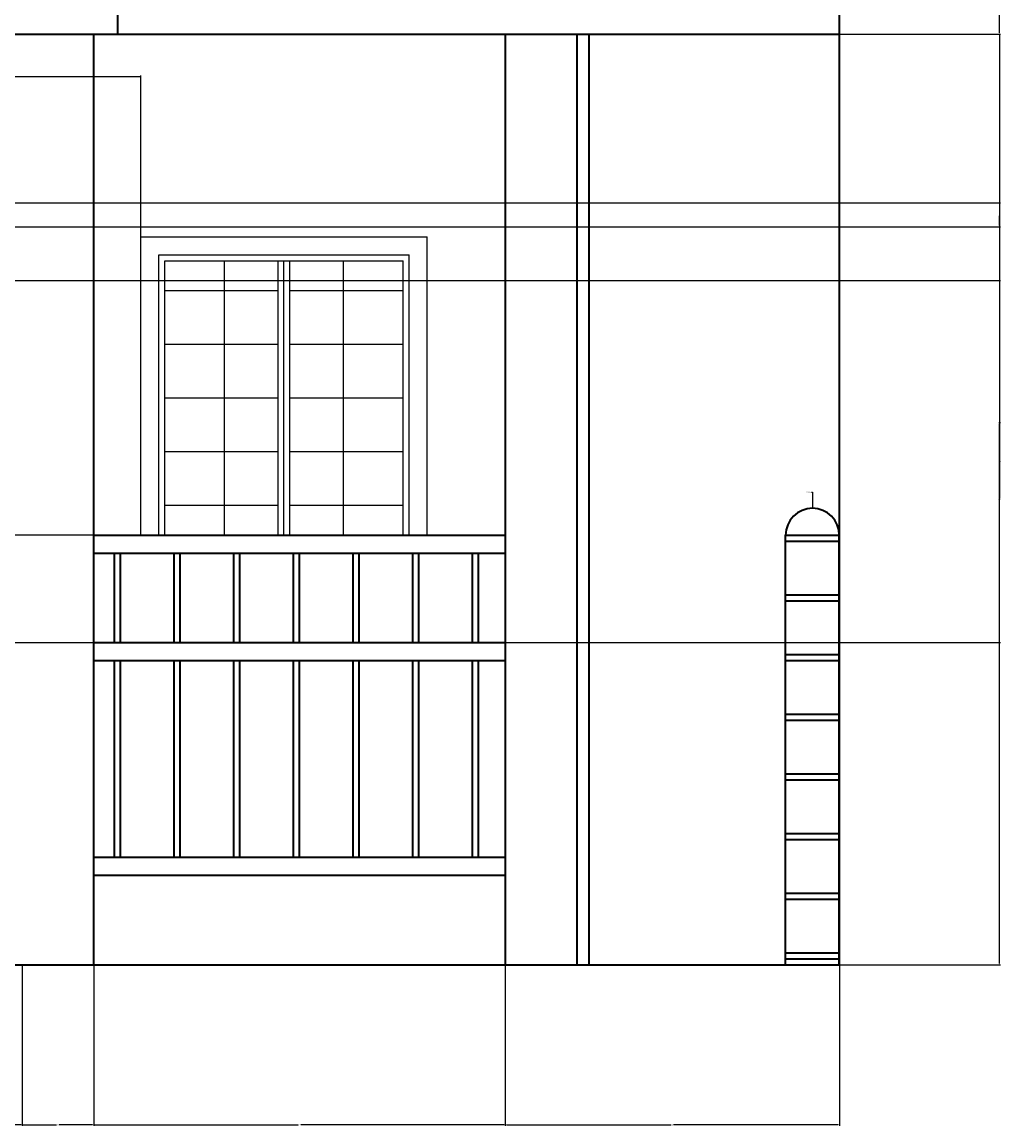
# Model space of a CAD drawing. Units: inches. Extents: x 2154 to 2740, y 571 to 1084.
# Tile 7 of 13: x 2576 to 2740, y 571 to 756. Entities that reach past the tile are written whole.
import ezdxf

# ---------------------------------------------------------------- set-up
doc = ezdxf.new("R2010")
doc.units = ezdxf.units.IN
for name, color, linetype, lineweight in [('A-ANNO-DIMS', 2, 'Continuous', 18), ('A-ELEV', 7, 'Continuous', 35), ('A-GLAZ', 4, 'Continuous', 25)]:
    doc.layers.add(name, color=color, linetype=linetype, lineweight=lineweight)
doc.styles.get("Standard").update_dxf_attribs({"font": 'arial.ttf'})
doc.dimstyles.get("Standard").update_dxf_attribs({"dimtxt": 0.18, "dimasz": 0.18, "dimexe": 0.18, "dimexo": 0.0625, "dimgap": 0.09, "dimtad": 0, "dimtih": 1, "dimtoh": 1, "dimdec": 4, "dimzin": 0, "dimdsep": 46, "dimtxsty": 'Standard', "dimcen": 0.09, "dimadec": 0, "dimazin": 0, "dimtfac": 1, "dimtdec": 4, "dimtofl": 0, "dimtmove": 0, "dimatfit": 3, "dimfxl": 1, "dimtolj": 1, "dimtzin": 0, "dimarcsym": 0})

# ---------------------------------------------------------------- blocks, each defined once
blk = doc.blocks.new('WIN-ELEV-1200')
for p, q in [((0, 50), (48, 50)), ((0, 0), (0, 50)), ((48, 0), (48, 50)), ((3, 0), (3, 47)), ((3, 47), (45, 47)), ((45, 0), (45, 47)), ((4, 46), (44, 46)), ((4, 0), (4, 46)), ((14, 0), (14, 46)), ((23, 0), (23, 46)), ((24, 0), (24, 46)), ((25, 0), (25, 46)), ((34, 0), (34, 46)), ((44, 0), (44, 46)), ((4, 41), (23, 41)), ((25, 41), (44, 41)), ((4, 32), (23, 32)), ((25, 32), (44, 32)), ((4, 23), (23, 23)), ((25, 23), (44, 23)), ((4, 14), (23, 14)), ((25, 14), (44, 14)), ((4, 5), (23, 5)), ((25, 5), (44, 5))]:
    blk.add_line(p, q)
blk = doc.blocks.new('*D11')
at = {"layer": 'A-ANNO-DIMS', "color": 0, "lineweight": -2, "transparency": 16777216}
for p, q in [((2713.27, 753.53), (2740.24, 753.53)), ((2740.06, 753.35), (2740.06, 675.71)), ((2740.06, 597.71), (2740.06, 675.35)), ((2713.27, 597.53), (2740.24, 597.53))]:
    blk.add_line(p, q, dxfattribs=at)
at = {"layer": 'A-ANNO-DIMS', "color": 0, "transparency": 16777216}
for points in [[(2740.03, 753.35), (2740.09, 753.35), (2740.06, 753.53)], [(2740.03, 597.71), (2740.09, 597.71), (2740.06, 597.53)]]:
    blk.add_solid(points, dxfattribs=at)
at = {"layer": 'Defpoints', "color": 0, "transparency": 16777216}
for p in [(2713.21, 753.53), (2740.06, 753.53), (2713.21, 597.53)]:
    blk.add_point(p, dxfattribs=at)
at = {"layer": 'A-ANNO-DIMS', "color": 0, "transparency": 16777216, "insert": (2740.06, 675.53), "char_height": 0.18, "attachment_point": 5}
blk.add_mtext('\\A1;156', dxfattribs=at)
blk = doc.blocks.new('*D12')
at = {"layer": 'A-ANNO-DIMS', "color": 0, "lineweight": -2, "transparency": 16777216}
for p, q in [((2713.27, 981.53), (2740.24, 981.53)), ((2740.06, 981.35), (2740.06, 867.71)), ((2740.06, 753.71), (2740.06, 867.35)), ((2713.27, 753.53), (2740.24, 753.53))]:
    blk.add_line(p, q, dxfattribs=at)
at = {"layer": 'A-ANNO-DIMS', "color": 0, "transparency": 16777216}
for points in [[(2740.03, 981.35), (2740.09, 981.35), (2740.06, 981.53)], [(2740.03, 753.71), (2740.09, 753.71), (2740.06, 753.53)]]:
    blk.add_solid(points, dxfattribs=at)
at = {"layer": 'Defpoints', "color": 0, "transparency": 16777216}
for p in [(2713.21, 981.53), (2740.06, 981.53), (2713.21, 753.53)]:
    blk.add_point(p, dxfattribs=at)
at = {"layer": 'A-ANNO-DIMS', "color": 0, "transparency": 16777216, "insert": (2740.06, 867.53), "char_height": 0.18, "attachment_point": 5}
blk.add_mtext('\\A1;228', dxfattribs=at)
blk = doc.blocks.new('*D25')
at = {"layer": 'A-ANNO-DIMS', "color": 0, "lineweight": -2, "transparency": 16777216}
for p, q in [((2507.21, 597.47), (2507.21, 570.5)), ((2576.21, 597.47), (2576.21, 570.5)), ((2507.39, 570.68), (2541.49, 570.68)), ((2576.03, 570.68), (2541.93, 570.68))]:
    blk.add_line(p, q, dxfattribs=at)
at = {"layer": 'A-ANNO-DIMS', "color": 0, "transparency": 16777216}
for points in [[(2507.39, 570.71), (2507.39, 570.65), (2507.21, 570.68)], [(2576.03, 570.71), (2576.03, 570.65), (2576.21, 570.68)]]:
    blk.add_solid(points, dxfattribs=at)
at = {"layer": 'Defpoints', "color": 0, "transparency": 16777216}
for p in [(2507.21, 597.53), (2576.21, 597.53), (2576.21, 570.68)]:
    blk.add_point(p, dxfattribs=at)
at = {"layer": 'A-ANNO-DIMS', "color": 0, "transparency": 16777216, "insert": (2541.71, 570.68), "char_height": 0.18, "attachment_point": 5}
blk.add_mtext('\\A1;69', dxfattribs=at)
blk = doc.blocks.new('*D26')
at = {"layer": 'A-ANNO-DIMS', "color": 0, "lineweight": -2, "transparency": 16777216}
for p, q in [((2576.21, 597.47), (2576.21, 570.5)), ((2588.21, 597.47), (2588.21, 570.5)), ((2576.39, 570.68), (2582, 570.68)), ((2588.03, 570.68), (2582.42, 570.68))]:
    blk.add_line(p, q, dxfattribs=at)
at = {"layer": 'A-ANNO-DIMS', "color": 0, "transparency": 16777216}
for points in [[(2576.39, 570.71), (2576.39, 570.65), (2576.21, 570.68)], [(2588.03, 570.71), (2588.03, 570.65), (2588.21, 570.68)]]:
    blk.add_solid(points, dxfattribs=at)
at = {"layer": 'Defpoints', "color": 0, "transparency": 16777216}
for p in [(2576.21, 597.53), (2588.21, 597.53), (2588.21, 570.68)]:
    blk.add_point(p, dxfattribs=at)
at = {"layer": 'A-ANNO-DIMS', "color": 0, "transparency": 16777216, "insert": (2582.21, 570.68), "char_height": 0.18, "attachment_point": 5}
blk.add_mtext('\\A1;12', dxfattribs=at)
blk = doc.blocks.new('*D27')
at = {"layer": 'A-ANNO-DIMS', "color": 0, "lineweight": -2, "transparency": 16777216}
for p, q in [((2588.21, 597.47), (2588.21, 570.5)), ((2657.21, 597.47), (2657.21, 570.5)), ((2588.39, 570.68), (2622.49, 570.68)), ((2657.03, 570.68), (2622.93, 570.68))]:
    blk.add_line(p, q, dxfattribs=at)
at = {"layer": 'A-ANNO-DIMS', "color": 0, "transparency": 16777216}
for points in [[(2588.39, 570.71), (2588.39, 570.65), (2588.21, 570.68)], [(2657.03, 570.71), (2657.03, 570.65), (2657.21, 570.68)]]:
    blk.add_solid(points, dxfattribs=at)
at = {"layer": 'Defpoints', "color": 0, "transparency": 16777216}
for p in [(2588.21, 597.53), (2657.21, 597.53), (2657.21, 570.68)]:
    blk.add_point(p, dxfattribs=at)
at = {"layer": 'A-ANNO-DIMS', "color": 0, "transparency": 16777216, "insert": (2622.71, 570.68), "char_height": 0.18, "attachment_point": 5}
blk.add_mtext('\\A1;69', dxfattribs=at)
blk = doc.blocks.new('*D28')
at = {"layer": 'A-ANNO-DIMS', "color": 0, "lineweight": -2, "transparency": 16777216}
for p, q in [((2657.21, 597.47), (2657.21, 570.5)), ((2713.21, 597.47), (2713.21, 570.5)), ((2657.39, 570.68), (2684.99, 570.68)), ((2713.03, 570.68), (2685.43, 570.68))]:
    blk.add_line(p, q, dxfattribs=at)
at = {"layer": 'A-ANNO-DIMS', "color": 0, "transparency": 16777216}
for points in [[(2657.39, 570.71), (2657.39, 570.65), (2657.21, 570.68)], [(2713.03, 570.71), (2713.03, 570.65), (2713.21, 570.68)]]:
    blk.add_solid(points, dxfattribs=at)
at = {"layer": 'Defpoints', "color": 0, "transparency": 16777216}
for p in [(2657.21, 597.53), (2713.21, 597.53), (2713.21, 570.68)]:
    blk.add_point(p, dxfattribs=at)
at = {"layer": 'A-ANNO-DIMS', "color": 0, "transparency": 16777216, "insert": (2685.21, 570.68), "char_height": 0.18, "attachment_point": 5}
blk.add_mtext('\\A1;56', dxfattribs=at)
blk = doc.blocks.new('*D29')
at = {"layer": 'A-ANNO-DIMS', "color": 0, "lineweight": -2, "transparency": 16777216}
for p, q in [((2657.14, 669.53), (2154.18, 669.53)), ((2154.36, 669.35), (2154.36, 633.71)), ((2154.36, 597.71), (2154.36, 633.35)), ((2657.14, 597.53), (2154.18, 597.53))]:
    blk.add_line(p, q, dxfattribs=at)
at = {"layer": 'A-ANNO-DIMS', "color": 0, "transparency": 16777216}
for points in [[(2154.33, 669.35), (2154.39, 669.35), (2154.36, 669.53)], [(2154.33, 597.71), (2154.39, 597.71), (2154.36, 597.53)]]:
    blk.add_solid(points, dxfattribs=at)
at = {"layer": 'Defpoints', "color": 0, "transparency": 16777216}
for p in [(2154.36, 669.53), (2657.21, 669.53), (2657.21, 597.53)]:
    blk.add_point(p, dxfattribs=at)
at = {"layer": 'A-ANNO-DIMS', "color": 0, "transparency": 16777216, "insert": (2154.36, 633.53), "char_height": 0.18, "attachment_point": 5}
blk.add_mtext('\\A1;72', dxfattribs=at)
blk = doc.blocks.new('*D45')
at = {"layer": 'A-ANNO-DIMS', "color": 0, "lineweight": -2, "transparency": 16777216}
for p, q in [((2515.25, 719.59), (2515.25, 746.56)), ((2515.43, 746.38), (2555.29, 746.38)), ((2595.93, 746.38), (2556.07, 746.38)), ((2596.11, 719.59), (2596.11, 746.56))]:
    blk.add_line(p, q, dxfattribs=at)
at = {"layer": 'A-ANNO-DIMS', "color": 0, "transparency": 16777216}
for points in [[(2515.43, 746.41), (2515.43, 746.35), (2515.25, 746.38)], [(2595.93, 746.41), (2595.93, 746.35), (2596.11, 746.38)]]:
    blk.add_solid(points, dxfattribs=at)
at = {"layer": 'Defpoints', "color": 0, "transparency": 16777216}
for p in [(2596.11, 746.38), (2515.25, 719.53), (2596.11, 719.53)]:
    blk.add_point(p, dxfattribs=at)
at = {"layer": 'A-ANNO-DIMS', "color": 0, "transparency": 16777216, "insert": (2555.68, 746.38), "char_height": 0.18, "attachment_point": 5}
blk.add_mtext('\\A1;80.86', dxfattribs=at)
blk = doc.blocks.new('*D88')
at = {"layer": 'A-ANNO-DIMS', "color": 0, "lineweight": -2, "transparency": 16777216}
for p, q in [((2463.769199, 725.228066), (2740.236699, 725.228066)), ((2740.056699, 725.048066), (2740.056699, 723.408066)), ((2740.056699, 721.408066), (2740.056699, 723.048066)), ((2459.769199, 721.228066), (2740.236699, 721.228066))]:
    blk.add_line(p, q, dxfattribs=at)
at = {"layer": 'A-ANNO-DIMS', "color": 0, "transparency": 16777216}
for points in [[(2740.026699, 725.048066), (2740.086699, 725.048066), (2740.056699, 725.228066)], [(2740.026699, 721.408066), (2740.086699, 721.408066), (2740.056699, 721.228066)]]:
    blk.add_solid(points, dxfattribs=at)
at = {"layer": 'Defpoints', "color": 0, "transparency": 16777216}
for p in [(2463.706699, 725.228066), (2740.056699, 725.228066), (2459.706699, 721.228066)]:
    blk.add_point(p, dxfattribs=at)
at = {"layer": 'A-ANNO-DIMS', "color": 0, "transparency": 16777216, "insert": (2740.056699, 723.228066), "char_height": 0.18, "attachment_point": 5}
blk.add_mtext('\\A1;4', dxfattribs=at)
blk = doc.blocks.new('*D91')
at = {"layer": 'A-ANNO-DIMS', "color": 0, "lineweight": -2, "transparency": 16777216}
for p, q in [((2450.77, 712.23), (2740.24, 712.23)), ((2740.06, 712.05), (2740.06, 682.06)), ((2740.06, 651.71), (2740.06, 681.7)), ((2450.77, 651.53), (2740.24, 651.53))]:
    blk.add_line(p, q, dxfattribs=at)
at = {"layer": 'A-ANNO-DIMS', "color": 0, "transparency": 16777216}
for points in [[(2740.03, 712.05), (2740.09, 712.05), (2740.06, 712.23)], [(2740.03, 651.71), (2740.09, 651.71), (2740.06, 651.53)]]:
    blk.add_solid(points, dxfattribs=at)
at = {"layer": 'Defpoints', "color": 0, "transparency": 16777216}
for p in [(2450.71, 712.23), (2740.06, 712.23), (2450.71, 651.53)]:
    blk.add_point(p, dxfattribs=at)
at = {"layer": 'A-ANNO-DIMS', "color": 0, "transparency": 16777216, "insert": (2740.06, 681.88), "char_height": 0.18, "attachment_point": 5}
blk.add_mtext('\\A1;60.7', dxfattribs=at)
blk = doc.blocks.new('*D92')
at = {"layer": 'A-ANNO-DIMS', "color": 0, "lineweight": -2, "transparency": 16777216}
for p, q in [((2463.77, 725.23), (2740.24, 725.23)), ((2740.06, 725.05), (2740.06, 688.56)), ((2740.06, 651.71), (2740.06, 688.2)), ((2463.77, 651.53), (2740.24, 651.53))]:
    blk.add_line(p, q, dxfattribs=at)
at = {"layer": 'A-ANNO-DIMS', "color": 0, "transparency": 16777216}
for points in [[(2740.03, 725.05), (2740.09, 725.05), (2740.06, 725.23)], [(2740.03, 651.71), (2740.09, 651.71), (2740.06, 651.53)]]:
    blk.add_solid(points, dxfattribs=at)
at = {"layer": 'Defpoints', "color": 0, "transparency": 16777216}
for p in [(2463.71, 725.23), (2740.06, 725.23), (2463.71, 651.53)]:
    blk.add_point(p, dxfattribs=at)
at = {"layer": 'A-ANNO-DIMS', "color": 0, "transparency": 16777216, "insert": (2740.06, 688.38), "char_height": 0.18, "attachment_point": 5}
blk.add_mtext('\\A1;73.7', dxfattribs=at)
blk = doc.blocks.new('*D138')
at = {"layer": 'A-ANNO-DIMS', "color": 0, "lineweight": -2, "transparency": 16777216}
for p, q in [((2708.52, 676.73), (2708.7, 676.73)), ((2708.7, 676.73), (2708.7, 674.21)), ((2708.62, 669.53), (2708.8, 669.53)), ((2708.71, 669.44), (2708.71, 669.62))]:
    blk.add_line(p, q, dxfattribs=at)
at = {"layer": 'A-ANNO-DIMS', "color": 0, "transparency": 16777216}
blk.add_solid([(2708.73, 674.21), (2708.67, 674.21), (2708.7, 674.03)], dxfattribs=at)
at = {"layer": 'Defpoints', "color": 0, "transparency": 16777216}
for p in [(2708.7, 674.03), (2708.71, 669.53)]:
    blk.add_point(p, dxfattribs=at)
at = {"layer": 'A-ANNO-DIMS', "color": 0, "transparency": 16777216, "insert": (2707.99, 676.73), "char_height": 0.18, "attachment_point": 5}
blk.add_mtext('\\A1;6X R4.5', dxfattribs=at)

msp = doc.modelspace()

# ---------------------------------------------------------------- linework, layer by layer
at = {"layer": 'A-ELEV'}
for p, q in [((2713.2067, 981.5321), (2713.2067, 753.5321)), ((2592.2067, 777.5321), (2592.2067, 753.5321)), ((2181.2067, 753.5321), (2713.2067, 753.5321)), ((2588.2067, 753.5321), (2588.2067, 597.5321)), ((2657.2067, 753.5321), (2657.2067, 597.5321)), ((2669.2067, 753.5321), (2669.2067, 597.5321)), ((2671.2067, 753.5321), (2671.2067, 597.5321)), ((2713.2067, 753.5321), (2713.2067, 597.5321)), ((2588.2067, 669.5321), (2657.2067, 669.5321)), ((2704.2067, 597.5321), (2704.2067, 669.5321)), ((2704.2067, 669.5321), (2713.2067, 669.5321)), ((2704.2067, 668.5321), (2713.2067, 668.5321)), ((2713.2067, 597.5321), (2713.2067, 669.5321)), ((2588.2067, 666.5321), (2657.2067, 666.5321)), ((2591.6527, 666.5321), (2591.6527, 651.5321)), ((2592.6527, 666.5321), (2592.6527, 651.5321)), ((2601.6527, 666.5321), (2601.6527, 651.5321)), ((2602.6527, 666.5321), (2602.6527, 651.5321)), ((2611.6527, 666.5321), (2611.6527, 651.5321)), ((2612.6527, 666.5321), (2612.6527, 651.5321)), ((2621.6527, 666.5321), (2621.6527, 651.5321)), ((2622.6527, 666.5321), (2622.6527, 651.5321)), ((2631.6527, 666.5321), (2631.6527, 651.5321)), ((2632.6527, 666.5321), (2632.6527, 651.5321)), ((2641.6527, 666.5321), (2641.6527, 651.5321)), ((2642.6527, 666.5321), (2642.6527, 651.5321)), ((2651.6527, 666.5321), (2651.6527, 651.5321)), ((2652.6527, 666.5321), (2652.6527, 651.5321)), ((2704.2067, 659.5321), (2713.2067, 659.5321)), ((2704.2067, 658.5321), (2713.2067, 658.5321)), ((2588.2067, 651.5321), (2657.2067, 651.5321)), ((2704.2067, 649.5321), (2713.2067, 649.5321)), ((2588.2067, 648.5321), (2657.2067, 648.5321)), ((2591.6527, 648.5321), (2591.6527, 615.5321)), ((2592.6527, 648.5321), (2592.6527, 615.5321)), ((2601.6527, 648.5321), (2601.6527, 615.5321)), ((2602.6527, 648.5321), (2602.6527, 615.5321)), ((2611.6527, 648.5321), (2611.6527, 615.5321)), ((2612.6527, 648.5321), (2612.6527, 615.5321)), ((2621.6527, 648.5321), (2621.6527, 615.5321)), ((2622.6527, 648.5321), (2622.6527, 615.5321)), ((2631.6527, 648.5321), (2631.6527, 615.5321)), ((2632.6527, 648.5321), (2632.6527, 615.5321)), ((2641.6527, 648.5321), (2641.6527, 615.5321)), ((2642.6527, 648.5321), (2642.6527, 615.5321)), ((2651.6527, 648.5321), (2651.6527, 615.5321)), ((2652.6527, 648.5321), (2652.6527, 615.5321)), ((2704.2067, 648.5321), (2713.2067, 648.5321)), ((2704.2067, 639.5321), (2713.2067, 639.5321)), ((2704.2067, 638.5321), (2713.2067, 638.5321)), ((2704.2067, 629.5321), (2713.2067, 629.5321)), ((2704.2067, 628.5321), (2713.2067, 628.5321)), ((2704.2067, 619.5321), (2713.2067, 619.5321)), ((2704.2067, 618.5321), (2713.2067, 618.5321)), ((2588.2067, 615.5321), (2657.2067, 615.5321)), ((2588.2067, 612.5321), (2657.2067, 612.5321)), ((2704.2067, 609.5321), (2713.2067, 609.5321)), ((2704.2067, 608.5321), (2713.2067, 608.5321)), ((2704.2067, 599.5321), (2713.2067, 599.5321)), ((2704.2067, 598.5321), (2713.2067, 598.5321)), ((2183.2067, 597.5321), (2713.2067, 597.5321)), ((2223.2067, 597.5321), (2671.2067, 597.5321))]:
    msp.add_line(p, q, dxfattribs=at)
msp.add_arc((2708.7067, 669.5321), 4.5, 0, 180, dxfattribs=at)

# ---------------------------------------------------------------- block references
at = {"layer": 'A-GLAZ'}
msp.add_blockref('WIN-ELEV-1200', (2596.1121, 669.532), dxfattribs=at)

# ---------------------------------------------------------------- dimensions: what is measured, and where the dimension line sits
at = {"layer": 'A-ANNO-DIMS'}
for base, p1, p2, angle, override, picture, middle in [((2740.0567, 981.5321), (2713.2067, 753.5321), (2713.2067, 981.5321), 90, {"dimdec": 0, "dimlfac": 1, "dimrnd": 0, "dimzin": 0, "dimdsep": 46, "dimlunit": 2}, '*D12', (2740.0567, 867.5321)), ((2740.0567, 753.5321), (2713.2067, 597.5321), (2713.2067, 753.5321), 90, {"dimdec": 0, "dimlfac": 1, "dimrnd": 0, "dimzin": 0, "dimdsep": 46, "dimlunit": 2}, '*D11', (2740.0567, 675.5321)), ((2596.1118, 746.3821), (2515.2489, 719.5321), (2596.1118, 719.5321), 0, {"dimdec": 2, "dimlfac": 1, "dimrnd": 0, "dimzin": 0, "dimdsep": 46, "dimlunit": 2}, '*D45', (2555.6803, 746.3821)), ((2740.0567, 725.2281), (2459.7067, 721.2281), (2463.7067, 725.2281), 90, {"dimdec": 0, "dimlfac": 1, "dimrnd": 0, "dimzin": 0, "dimdsep": 46, "dimlunit": 2}, '*D88', (2740.0567, 723.2281)), ((2740.0567, 725.2281), (2463.7067, 651.5321), (2463.7067, 725.2281), 90, {"dimdec": 1, "dimlfac": 1, "dimrnd": 0, "dimzin": 0, "dimdsep": 46, "dimlunit": 2}, '*D92', (2740.0567, 688.3801)), ((2740.0567, 712.2281), (2450.7067, 651.5321), (2450.7067, 712.2281), 90, {"dimdec": 1, "dimlfac": 1, "dimrnd": 0, "dimzin": 0, "dimdsep": 46, "dimlunit": 2}, '*D91', (2740.0567, 681.8801)), ((2154.3567, 669.5321), (2657.2067, 597.5321), (2657.2067, 669.5321), 90, {"dimdec": 0, "dimlfac": 1, "dimrnd": 0, "dimzin": 0, "dimdsep": 46, "dimlunit": 2}, '*D29', (2154.3567, 633.5321))]:
    dim = msp.add_linear_dim(base=base, p1=p1, p2=p2, angle=angle, dimstyle='Standard', override=override, dxfattribs=at)
    dim.commit()
    dim.dimension.update_dxf_attribs({"geometry": picture, "text_midpoint": middle})
dim = msp.add_radius_dim(center=(2708.7067, 669.5321), mpoint=(2708.7033, 674.0321), text='6X <>', dimstyle='Standard', override={"dimdec": 1, "dimlfac": 1, "dimrnd": 0, "dimzin": 0, "dimdsep": 46, "dimlunit": 2}, dxfattribs=at)
dim.commit()
dim.dimension.update_dxf_attribs({"geometry": '*D138', "text_midpoint": (2707.9868, 676.7321), "dimtype": 164})
for base, p1, p2, picture, middle in [((2576.2067, 570.6821), (2507.2067, 597.5321), (2576.2067, 597.5321), '*D25', (2541.7067, 570.6821)), ((2588.2067, 570.6821), (2576.2067, 597.5321), (2588.2067, 597.5321), '*D26', (2582.2067, 570.6821)), ((2657.2067, 570.6821), (2588.2067, 597.5321), (2657.2067, 597.5321), '*D27', (2622.7067, 570.6821)), ((2713.2067, 570.6821), (2657.2067, 597.5321), (2713.2067, 597.5321), '*D28', (2685.2067, 570.6821))]:
    dim = msp.add_linear_dim(base=base, p1=p1, p2=p2, dimstyle='Standard', override={"dimdec": 0, "dimlfac": 1, "dimrnd": 0, "dimzin": 0, "dimdsep": 46, "dimlunit": 2}, dxfattribs=at)
    dim.commit()
    dim.dimension.update_dxf_attribs({"geometry": picture, "text_midpoint": middle})

doc.saveas('drawing.dxf')
